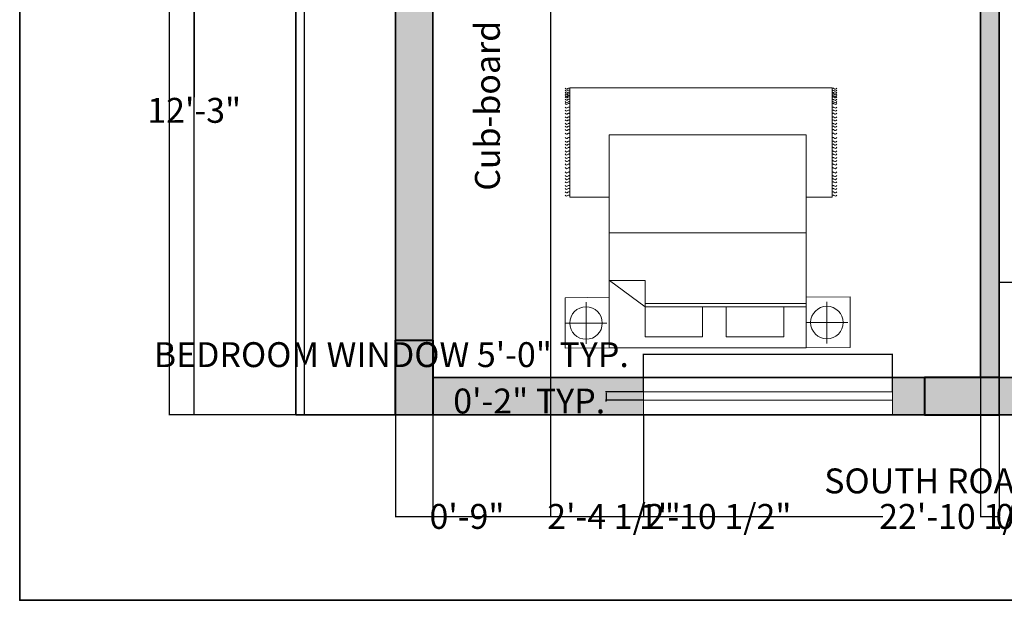
# Model space of a CAD drawing. Units: inches. Extents: x 56944 to 57417, y 173916 to 174454.
# Tile 1 of 8: x 56944 to 57181, y 173916 to 174056. Entities that reach past the tile are written whole.
import ezdxf

# ---------------------------------------------------------------- set-up
doc = ezdxf.new("R2010")
doc.units = ezdxf.units.IN
doc.header["$MEASUREMENT"] = 0
for name, color, linetype, lineweight in [('A-ANNO-DIMS', 2, 'Continuous', 18), ('A-ANNO-TEXT', 7, 'Continuous', 18), ('A-ANNO-TTLB', 7, 'Continuous', 35), ('A-COLS', 7, 'Continuous', 40), ('A-COLS-PATT', 250, 'Continuous', 9), ('A-FLOR-CASE', 8, 'Continuous', 25), ('A-FURN', 8, 'Continuous', 18), ('A-GLAZ', 4, 'Continuous', 18), ('A-SITE-PATT', 8, 'Continuous', 9), ('A-SITE-WALL', 7, 'Continuous', 25), ('A-WALL', 7, 'Continuous', 35), ('A-WALL-PATT', 241, 'Continuous', 9), ('C-PROP', 7, 'Continuous', 35)]:
    doc.layers.add(name, color=color, linetype=linetype, lineweight=lineweight)
doc.styles.get("Standard").update_dxf_attribs({"font": 'arial.ttf'})
doc.dimstyles.get("Standard").update_dxf_attribs({"dimtxt": 6, "dimasz": 0.18, "dimexe": 0.18, "dimexo": 0.0625, "dimgap": 0.09, "dimtad": 0, "dimtih": 1, "dimtoh": 1, "dimdec": 1, "dimzin": 0, "dimdsep": 46, "dimlunit": 3, "dimtxsty": 'Standard', "dimcen": 0.09, "dimadec": 0, "dimazin": 0, "dimtfac": 1, "dimtdec": 1, "dimtofl": 0, "dimtmove": 0, "dimatfit": 3, "dimfxl": 1, "dimtolj": 1, "dimtzin": 0, "dimarcsym": 0})

# ---------------------------------------------------------------- blocks, each defined once
blk = doc.blocks.new('*D4')
at = {"layer": 'A-ANNO-DIMS', "color": 0, "lineweight": -2, "transparency": 16777216}
for p, q in [((57010.07, 174399.82), (56979.48, 174399.82)), ((56979.66, 174399.64), (56979.66, 174183.23)), ((56979.66, 173960.5), (56979.66, 174176.92)), ((57010.07, 173960.32), (56979.48, 173960.32))]:
    blk.add_line(p, q, dxfattribs=at)
at = {"layer": 'A-ANNO-DIMS', "color": 0, "transparency": 16777216}
for points in [[(56979.63, 174399.64), (56979.69, 174399.64), (56979.66, 174399.82)], [(56979.63, 173960.5), (56979.69, 173960.5), (56979.66, 173960.32)]]:
    blk.add_solid(points, dxfattribs=at)
at = {"layer": 'Defpoints', "color": 0, "transparency": 16777216}
for p in [(57010.13, 174399.82), (56979.66, 173960.32), (57010.13, 173960.32)]:
    blk.add_point(p, dxfattribs=at)
at = {"layer": 'A-ANNO-DIMS', "color": 0, "transparency": 16777216, "insert": (56979.66, 174180.07), "char_height": 6, "width": 27.5975, "attachment_point": 5}
blk.add_mtext("\\A1;40'", dxfattribs=at)
blk = doc.blocks.new('BED-DOUBLE-WITH-NIGHTSTANDS')
for p, q in [((6.09, 68.68), (6.09, 58.62)), ((36.42, 67.59), (62.78, 67.59)), ((36.42, 58.05), (36.42, 67.59)), ((62.78, 67.59), (62.78, 4.35)), ((1.07, 63.65), (11.12, 63.65)), ((9.97, 49.39), (16.32, 58)), ((16.32, 49.44), (16.32, 58)), ((27.82, 58.05), (27.82, 10.63)), ((9.97, 49.44), (16.32, 49.44)), ((9.97, 49.39), (9.97, 10.63)), ((10.78, 49.44), (10.78, 10.63)), ((6.2, 10.63), (6.2, 0.57)), ((36.42, 4.35), (36.42, 10.65)), ((1.17, 5.6), (11.22, 5.6)), ((62.78, 4.35), (36.42, 4.35))]:
    blk.add_line(p, q)
for points in [[(12.29, 58.05), (12.19, 68.68), (0, 68.68), (0.1, 58.05)], [(0.1, 58.05), (51.42, 58.05), (51.42, 10.63), (0.1, 10.63)], [(2.8, 49.44), (9.97, 49.44), (9.97, 35.55), (2.8, 35.55)], [(2.8, 29.88), (9.97, 29.88), (9.97, 15.98), (2.8, 15.98)], [(12.39, 0), (12.29, 10.63), (0.1, 10.63), (0.21, 0)]]:
    blk.add_lwpolyline(points, close=True)
for centre in [(6.09, 63.65), (6.2, 5.6)]:
    blk.add_circle(centre, 3.92)
for points, knots in [([(36.95, 68.71), (36.83, 68.61), (36.59, 68.42), (36.83, 68.08), (37, 67.8), (36.89, 67.65), (36.85, 67.58)], [0, 0, 0, 0, 0.400747, 0.791423, 1.067667, 1.29709, 1.29709, 1.29709, 1.29709]), ([(37.73, 68.71), (37.61, 68.61), (37.37, 68.42), (37.61, 68.08), (37.78, 67.8), (37.67, 67.65), (37.62, 67.58)], [0, 0, 0, 0, 0.400747, 0.791423, 1.067667, 1.29709, 1.29709, 1.29709, 1.29709]), ([(38.54, 68.71), (38.42, 68.61), (38.18, 68.42), (38.42, 68.08), (38.59, 67.8), (38.49, 67.65), (38.44, 67.58)], [0, 0, 0, 0, 0.400747, 0.791423, 1.067667, 1.29709, 1.29709, 1.29709, 1.29709]), ([(39.27, 68.71), (39.15, 68.61), (38.91, 68.42), (39.15, 68.08), (39.32, 67.8), (39.22, 67.65), (39.17, 67.58)], [0, 0, 0, 0, 0.400747, 0.791423, 1.067667, 1.29709, 1.29709, 1.29709, 1.29709]), ([(40.15, 68.71), (40.03, 68.61), (39.79, 68.42), (40.03, 68.08), (40.2, 67.8), (40.1, 67.65), (40.05, 67.58)], [0, 0, 0, 0, 0.400747, 0.791423, 1.067667, 1.29709, 1.29709, 1.29709, 1.29709]), ([(40.91, 68.71), (40.78, 68.61), (40.54, 68.42), (40.78, 68.08), (40.96, 67.8), (40.85, 67.65), (40.8, 67.58)], [0, 0, 0, 0, 0.400747, 0.791423, 1.067667, 1.29709, 1.29709, 1.29709, 1.29709]), ([(41.63, 68.71), (41.51, 68.61), (41.27, 68.42), (41.51, 68.08), (41.68, 67.8), (41.58, 67.65), (41.53, 67.58)], [0, 0, 0, 0, 0.400747, 0.791423, 1.067667, 1.29709, 1.29709, 1.29709, 1.29709]), ([(42.52, 68.71), (42.39, 68.61), (42.15, 68.42), (42.39, 68.08), (42.57, 67.8), (42.46, 67.65), (42.41, 67.58)], [0, 0, 0, 0, 0.400747, 0.791423, 1.067667, 1.29709, 1.29709, 1.29709, 1.29709]), ([(43.55, 68.71), (43.43, 68.61), (43.19, 68.42), (43.43, 68.08), (43.6, 67.8), (43.5, 67.65), (43.45, 67.58)], [0, 0, 0, 0, 0.400747, 0.791423, 1.067667, 1.29709, 1.29709, 1.29709, 1.29709]), ([(44.43, 68.71), (44.31, 68.61), (44.07, 68.42), (44.31, 68.08), (44.49, 67.8), (44.38, 67.65), (44.33, 67.58)], [0, 0, 0, 0, 0.400747, 0.791423, 1.067667, 1.29709, 1.29709, 1.29709, 1.29709]), ([(45.25, 68.71), (45.13, 68.61), (44.89, 68.42), (45.13, 68.08), (45.3, 67.8), (45.2, 67.65), (45.15, 67.58)], [0, 0, 0, 0, 0.400747, 0.791423, 1.067667, 1.29709, 1.29709, 1.29709, 1.29709]), ([(46.03, 68.71), (45.91, 68.61), (45.67, 68.42), (45.91, 68.08), (46.08, 67.8), (45.97, 67.65), (45.92, 67.58)], [0, 0, 0, 0, 0.400747, 0.791423, 1.067667, 1.29709, 1.29709, 1.29709, 1.29709]), ([(46.84, 68.71), (46.72, 68.61), (46.48, 68.42), (46.72, 68.08), (46.9, 67.8), (46.79, 67.65), (46.74, 67.58)], [0, 0, 0, 0, 0.400747, 0.791423, 1.067667, 1.29709, 1.29709, 1.29709, 1.29709]), ([(47.57, 68.71), (47.45, 68.61), (47.21, 68.42), (47.45, 68.08), (47.62, 67.8), (47.52, 67.65), (47.47, 67.58)], [0, 0, 0, 0, 0.400747, 0.791423, 1.067667, 1.29709, 1.29709, 1.29709, 1.29709]), ([(48.45, 68.71), (48.33, 68.61), (48.09, 68.42), (48.33, 68.08), (48.51, 67.8), (48.4, 67.65), (48.35, 67.58)], [0, 0, 0, 0, 0.400747, 0.791423, 1.067667, 1.29709, 1.29709, 1.29709, 1.29709]), ([(49.21, 68.71), (49.08, 68.61), (48.85, 68.42), (49.08, 68.08), (49.26, 67.8), (49.15, 67.65), (49.1, 67.58)], [0, 0, 0, 0, 0.400747, 0.791423, 1.067667, 1.29709, 1.29709, 1.29709, 1.29709]), ([(49.93, 68.71), (49.81, 68.61), (49.57, 68.42), (49.81, 68.08), (49.99, 67.8), (49.88, 67.65), (49.83, 67.58)], [0, 0, 0, 0, 0.400747, 0.791423, 1.067667, 1.29709, 1.29709, 1.29709, 1.29709]), ([(50.82, 68.71), (50.69, 68.61), (50.46, 68.42), (50.69, 68.08), (50.87, 67.8), (50.76, 67.65), (50.71, 67.58)], [0, 0, 0, 0, 0.400747, 0.791423, 1.067667, 1.29709, 1.29709, 1.29709, 1.29709]), ([(51.85, 68.71), (51.73, 68.61), (51.49, 68.42), (51.73, 68.08), (51.9, 67.8), (51.8, 67.65), (51.75, 67.58)], [0, 0, 0, 0, 0.400747, 0.791423, 1.067667, 1.29709, 1.29709, 1.29709, 1.29709]), ([(52.73, 68.71), (52.61, 68.61), (52.37, 68.42), (52.61, 68.08), (52.79, 67.8), (52.68, 67.65), (52.63, 67.58)], [0, 0, 0, 0, 0.400747, 0.791423, 1.067667, 1.29709, 1.29709, 1.29709, 1.29709]), ([(53.55, 68.71), (53.43, 68.61), (53.19, 68.42), (53.43, 68.08), (53.6, 67.8), (53.5, 67.65), (53.45, 67.58)], [0, 0, 0, 0, 0.400747, 0.791423, 1.067667, 1.29709, 1.29709, 1.29709, 1.29709]), ([(54.24, 68.71), (54.12, 68.61), (53.88, 68.42), (54.12, 68.08), (54.29, 67.8), (54.19, 67.65), (54.14, 67.58)], [0, 0, 0, 0, 0.400747, 0.791423, 1.067667, 1.29709, 1.29709, 1.29709, 1.29709]), ([(55.06, 68.71), (54.94, 68.61), (54.7, 68.42), (54.94, 68.08), (55.11, 67.8), (55, 67.65), (54.95, 67.58)], [0, 0, 0, 0, 0.400747, 0.791423, 1.067667, 1.29709, 1.29709, 1.29709, 1.29709]), ([(55.78, 68.71), (55.66, 68.61), (55.42, 68.42), (55.66, 68.08), (55.84, 67.8), (55.73, 67.65), (55.68, 67.58)], [0, 0, 0, 0, 0.400747, 0.791423, 1.067667, 1.29709, 1.29709, 1.29709, 1.29709]), ([(56.67, 68.71), (56.55, 68.61), (56.31, 68.42), (56.55, 68.08), (56.72, 67.8), (56.61, 67.65), (56.56, 67.58)], [0, 0, 0, 0, 0.400747, 0.791423, 1.067667, 1.29709, 1.29709, 1.29709, 1.29709]), ([(57.42, 68.71), (57.3, 68.61), (57.06, 68.42), (57.3, 68.08), (57.47, 67.8), (57.36, 67.65), (57.32, 67.58)], [0, 0, 0, 0, 0.400747, 0.791423, 1.067667, 1.29709, 1.29709, 1.29709, 1.29709]), ([(58.15, 68.71), (58.03, 68.61), (57.79, 68.42), (58.03, 68.08), (58.2, 67.8), (58.1, 67.66), (58.05, 67.59)], [0, 0, 0, 0, 0.400747, 0.791423, 1.067667, 1.283686, 1.283686, 1.283686, 1.283686]), ([(59.03, 68.71), (58.91, 68.61), (58.67, 68.42), (58.91, 68.08), (59.08, 67.8), (58.98, 67.66), (58.93, 67.59)], [0, 0, 0, 0, 0.400747, 0.791423, 1.067667, 1.283686, 1.283686, 1.283686, 1.283686]), ([(59.46, 68.71), (59.34, 68.61), (59.09, 68.42), (59.34, 68.08), (59.51, 67.8), (59.41, 67.66), (59.36, 67.59)], [0, 0, 0, 0, 0.402903, 0.794912, 1.071156, 1.287177, 1.287177, 1.287177, 1.287177]), ([(60.05, 68.71), (59.93, 68.61), (59.69, 68.42), (59.93, 68.08), (60.1, 67.8), (60, 67.66), (59.96, 67.59)], [0, 0, 0, 0, 0.400747, 0.791423, 1.067667, 1.283686, 1.283686, 1.283686, 1.283686]), ([(60.63, 68.71), (60.51, 68.61), (60.27, 68.42), (60.51, 68.08), (60.68, 67.8), (60.58, 67.66), (60.53, 67.59)], [0, 0, 0, 0, 0.400747, 0.791423, 1.067667, 1.283686, 1.283686, 1.283686, 1.283686]), ([(60.94, 68.71), (60.82, 68.61), (60.58, 68.42), (60.81, 68.08), (60.99, 67.8), (60.89, 67.66), (60.84, 67.59)], [0, 0, 0, 0, 0.400747, 0.791423, 1.067667, 1.283686, 1.283686, 1.283686, 1.283686]), ([(61.35, 68.71), (61.23, 68.61), (60.99, 68.42), (61.23, 68.08), (61.41, 67.8), (61.3, 67.65), (61.25, 67.58)], [0, 0, 0, 0, 0.400747, 0.791423, 1.067667, 1.29709, 1.29709, 1.29709, 1.29709]), ([(61.75, 68.71), (61.63, 68.61), (61.39, 68.42), (61.63, 68.08), (61.8, 67.8), (61.7, 67.65), (61.65, 67.58)], [0, 0, 0, 0, 0.400747, 0.791423, 1.067667, 1.29709, 1.29709, 1.29709, 1.29709]), ([(62.24, 68.71), (62.12, 68.61), (61.88, 68.42), (62.12, 68.08), (62.29, 67.8), (62.18, 67.65), (62.13, 67.58)], [0, 0, 0, 0, 0.400747, 0.791423, 1.067667, 1.29709, 1.29709, 1.29709, 1.29709]), ([(62.71, 68.71), (62.59, 68.61), (62.35, 68.42), (62.59, 68.08), (62.76, 67.8), (62.66, 67.65), (62.61, 67.58)], [0, 0, 0, 0, 0.400747, 0.791423, 1.067667, 1.29709, 1.29709, 1.29709, 1.29709]), ([(36.95, 3.23), (36.83, 3.32), (36.59, 3.52), (36.83, 3.86), (37, 4.14), (36.89, 4.29), (36.85, 4.35)], [0, 0, 0, 0, 0.400747, 0.791423, 1.067667, 1.29709, 1.29709, 1.29709, 1.29709]), ([(37.73, 3.23), (37.61, 3.32), (37.37, 3.52), (37.61, 3.86), (37.78, 4.14), (37.67, 4.29), (37.62, 4.35)], [0, 0, 0, 0, 0.400747, 0.791423, 1.067667, 1.29709, 1.29709, 1.29709, 1.29709]), ([(38.54, 3.23), (38.42, 3.32), (38.18, 3.52), (38.42, 3.86), (38.59, 4.14), (38.49, 4.29), (38.44, 4.35)], [0, 0, 0, 0, 0.400747, 0.791423, 1.067667, 1.29709, 1.29709, 1.29709, 1.29709]), ([(39.27, 3.23), (39.15, 3.32), (38.91, 3.52), (39.15, 3.86), (39.32, 4.14), (39.22, 4.29), (39.17, 4.35)], [0, 0, 0, 0, 0.400747, 0.791423, 1.067667, 1.29709, 1.29709, 1.29709, 1.29709]), ([(40.15, 3.23), (40.03, 3.32), (39.79, 3.52), (40.03, 3.86), (40.2, 4.14), (40.1, 4.29), (40.05, 4.35)], [0, 0, 0, 0, 0.400747, 0.791423, 1.067667, 1.29709, 1.29709, 1.29709, 1.29709]), ([(40.91, 3.23), (40.78, 3.32), (40.54, 3.52), (40.78, 3.86), (40.96, 4.14), (40.85, 4.29), (40.8, 4.35)], [0, 0, 0, 0, 0.400747, 0.791423, 1.067667, 1.29709, 1.29709, 1.29709, 1.29709]), ([(41.63, 3.23), (41.51, 3.32), (41.27, 3.52), (41.51, 3.86), (41.68, 4.14), (41.58, 4.29), (41.53, 4.35)], [0, 0, 0, 0, 0.400747, 0.791423, 1.067667, 1.29709, 1.29709, 1.29709, 1.29709]), ([(42.52, 3.23), (42.39, 3.32), (42.15, 3.52), (42.39, 3.86), (42.57, 4.14), (42.46, 4.29), (42.41, 4.35)], [0, 0, 0, 0, 0.400747, 0.791423, 1.067667, 1.29709, 1.29709, 1.29709, 1.29709]), ([(43.55, 3.23), (43.43, 3.32), (43.19, 3.52), (43.43, 3.86), (43.6, 4.14), (43.5, 4.29), (43.45, 4.35)], [0, 0, 0, 0, 0.400747, 0.791423, 1.067667, 1.29709, 1.29709, 1.29709, 1.29709]), ([(44.43, 3.23), (44.31, 3.32), (44.07, 3.52), (44.31, 3.86), (44.49, 4.14), (44.38, 4.29), (44.33, 4.35)], [0, 0, 0, 0, 0.400747, 0.791423, 1.067667, 1.29709, 1.29709, 1.29709, 1.29709]), ([(45.25, 3.23), (45.13, 3.32), (44.89, 3.52), (45.13, 3.86), (45.3, 4.14), (45.2, 4.29), (45.15, 4.35)], [0, 0, 0, 0, 0.400747, 0.791423, 1.067667, 1.29709, 1.29709, 1.29709, 1.29709]), ([(46.03, 3.23), (45.91, 3.32), (45.67, 3.52), (45.91, 3.86), (46.08, 4.14), (45.97, 4.29), (45.92, 4.35)], [0, 0, 0, 0, 0.400747, 0.791423, 1.067667, 1.29709, 1.29709, 1.29709, 1.29709]), ([(46.84, 3.23), (46.72, 3.32), (46.48, 3.52), (46.72, 3.86), (46.9, 4.14), (46.79, 4.29), (46.74, 4.35)], [0, 0, 0, 0, 0.400747, 0.791423, 1.067667, 1.29709, 1.29709, 1.29709, 1.29709]), ([(47.57, 3.23), (47.45, 3.32), (47.21, 3.52), (47.45, 3.86), (47.62, 4.14), (47.52, 4.29), (47.47, 4.35)], [0, 0, 0, 0, 0.400747, 0.791423, 1.067667, 1.29709, 1.29709, 1.29709, 1.29709]), ([(48.45, 3.23), (48.33, 3.32), (48.09, 3.52), (48.33, 3.86), (48.51, 4.14), (48.4, 4.29), (48.35, 4.35)], [0, 0, 0, 0, 0.400747, 0.791423, 1.067667, 1.29709, 1.29709, 1.29709, 1.29709]), ([(49.21, 3.23), (49.08, 3.32), (48.85, 3.52), (49.08, 3.86), (49.26, 4.14), (49.15, 4.29), (49.1, 4.35)], [0, 0, 0, 0, 0.400747, 0.791423, 1.067667, 1.29709, 1.29709, 1.29709, 1.29709]), ([(49.93, 3.23), (49.81, 3.32), (49.57, 3.52), (49.81, 3.86), (49.99, 4.14), (49.88, 4.29), (49.83, 4.35)], [0, 0, 0, 0, 0.400747, 0.791423, 1.067667, 1.29709, 1.29709, 1.29709, 1.29709]), ([(50.82, 3.23), (50.69, 3.32), (50.46, 3.52), (50.69, 3.86), (50.87, 4.14), (50.76, 4.29), (50.71, 4.35)], [0, 0, 0, 0, 0.400747, 0.791423, 1.067667, 1.29709, 1.29709, 1.29709, 1.29709]), ([(51.85, 3.23), (51.73, 3.32), (51.49, 3.52), (51.73, 3.86), (51.9, 4.14), (51.8, 4.29), (51.75, 4.35)], [0, 0, 0, 0, 0.400747, 0.791423, 1.067667, 1.29709, 1.29709, 1.29709, 1.29709]), ([(52.73, 3.23), (52.61, 3.32), (52.37, 3.52), (52.61, 3.86), (52.79, 4.14), (52.68, 4.29), (52.63, 4.35)], [0, 0, 0, 0, 0.400747, 0.791423, 1.067667, 1.29709, 1.29709, 1.29709, 1.29709]), ([(53.55, 3.23), (53.43, 3.32), (53.19, 3.52), (53.43, 3.86), (53.6, 4.14), (53.5, 4.29), (53.45, 4.35)], [0, 0, 0, 0, 0.400747, 0.791423, 1.067667, 1.29709, 1.29709, 1.29709, 1.29709]), ([(54.24, 3.23), (54.12, 3.32), (53.88, 3.52), (54.12, 3.86), (54.29, 4.14), (54.19, 4.29), (54.14, 4.35)], [0, 0, 0, 0, 0.400747, 0.791423, 1.067667, 1.29709, 1.29709, 1.29709, 1.29709]), ([(55.06, 3.23), (54.94, 3.32), (54.7, 3.52), (54.94, 3.86), (55.11, 4.14), (55, 4.29), (54.95, 4.35)], [0, 0, 0, 0, 0.400747, 0.791423, 1.067667, 1.29709, 1.29709, 1.29709, 1.29709]), ([(55.78, 3.23), (55.66, 3.32), (55.42, 3.52), (55.66, 3.86), (55.84, 4.14), (55.73, 4.29), (55.68, 4.35)], [0, 0, 0, 0, 0.400747, 0.791423, 1.067667, 1.29709, 1.29709, 1.29709, 1.29709]), ([(56.67, 3.23), (56.55, 3.32), (56.31, 3.52), (56.55, 3.86), (56.72, 4.14), (56.61, 4.29), (56.56, 4.35)], [0, 0, 0, 0, 0.400747, 0.791423, 1.067667, 1.29709, 1.29709, 1.29709, 1.29709]), ([(57.42, 3.23), (57.3, 3.32), (57.06, 3.52), (57.3, 3.86), (57.47, 4.14), (57.36, 4.29), (57.32, 4.35)], [0, 0, 0, 0, 0.400747, 0.791423, 1.067667, 1.29709, 1.29709, 1.29709, 1.29709]), ([(58.15, 3.23), (58.03, 3.32), (57.79, 3.52), (58.03, 3.86), (58.2, 4.14), (58.09, 4.29), (58.04, 4.35)], [0, 0, 0, 0, 0.400747, 0.791423, 1.067667, 1.29709, 1.29709, 1.29709, 1.29709]), ([(59.03, 3.23), (58.91, 3.32), (58.67, 3.52), (58.91, 3.86), (59.08, 4.14), (58.97, 4.29), (58.93, 4.35)], [0, 0, 0, 0, 0.400747, 0.791423, 1.067667, 1.29709, 1.29709, 1.29709, 1.29709]), ([(59.46, 3.23), (59.33, 3.32), (59.08, 3.51), (59.34, 3.86), (59.51, 4.14), (59.4, 4.29), (59.36, 4.35)], [0, 0, 0, 0, 0.407265, 0.802015, 1.07826, 1.307683, 1.307683, 1.307683, 1.307683]), ([(60.03, 3.23), (59.9, 3.32), (59.67, 3.52), (59.9, 3.86), (60.08, 4.14), (59.97, 4.29), (59.92, 4.35)], [0, 0, 0, 0, 0.400747, 0.791423, 1.067667, 1.29709, 1.29709, 1.29709, 1.29709]), ([(60.6, 3.23), (60.48, 3.32), (60.24, 3.52), (60.48, 3.86), (60.65, 4.14), (60.54, 4.29), (60.5, 4.35)], [0, 0, 0, 0, 0.400747, 0.791423, 1.067667, 1.29709, 1.29709, 1.29709, 1.29709]), ([(60.91, 3.23), (60.79, 3.32), (60.55, 3.52), (60.79, 3.86), (60.96, 4.14), (60.85, 4.29), (60.81, 4.35)], [0, 0, 0, 0, 0.400747, 0.791423, 1.067667, 1.29709, 1.29709, 1.29709, 1.29709]), ([(61.33, 3.23), (61.21, 3.32), (60.97, 3.52), (61.21, 3.86), (61.38, 4.14), (61.27, 4.29), (61.22, 4.35)], [0, 0, 0, 0, 0.400747, 0.791423, 1.067667, 1.29709, 1.29709, 1.29709, 1.29709]), ([(61.72, 3.23), (61.6, 3.32), (61.36, 3.52), (61.6, 3.86), (61.78, 4.14), (61.67, 4.29), (61.62, 4.35)], [0, 0, 0, 0, 0.400747, 0.791423, 1.067667, 1.29709, 1.29709, 1.29709, 1.29709]), ([(62.21, 3.23), (62.09, 3.32), (61.85, 3.52), (62.09, 3.86), (62.26, 4.14), (62.15, 4.29), (62.11, 4.35)], [0, 0, 0, 0, 0.400747, 0.791423, 1.067667, 1.29709, 1.29709, 1.29709, 1.29709]), ([(62.71, 3.23), (62.59, 3.32), (62.35, 3.52), (62.59, 3.86), (62.76, 4.14), (62.66, 4.29), (62.61, 4.35)], [0, 0, 0, 0, 0.400747, 0.791423, 1.067667, 1.29709, 1.29709, 1.29709, 1.29709])]:
    blk.add_open_spline(points, degree=3, knots=knots)
blk = doc.blocks.new('GLAZ-LITE-60IN')
for p, q in [((0, 2), (60, 2)), ((60, 0), (0, 0))]:
    blk.add_line(p, q)
blk = doc.blocks.new('*D26')
at = {"layer": 'A-ANNO-DIMS', "color": 0, "lineweight": -2, "transparency": 16777216}
for p, q in [((57093.93, 173974.82), (57093.75, 173974.82)), ((57093.93, 173965.89), (57093.93, 173975)), ((57153.75, 173974.82), (57094.11, 173974.82)), ((57153.93, 173965.89), (57153.93, 173975))]:
    blk.add_line(p, q, dxfattribs=at)
at = {"layer": 'A-ANNO-DIMS', "color": 0, "transparency": 16777216}
for points in [[(57094.11, 173974.85), (57094.11, 173974.79), (57093.93, 173974.82)], [(57153.75, 173974.85), (57153.75, 173974.79), (57153.93, 173974.82)]]:
    blk.add_solid(points, dxfattribs=at)
at = {"layer": 'Defpoints', "color": 0, "transparency": 16777216}
for p in [(57093.93, 173974.82), (57093.93, 173965.82), (57153.93, 173965.82)]:
    blk.add_point(p, dxfattribs=at)
at = {"layer": 'A-ANNO-DIMS', "color": 0, "transparency": 16777216, "insert": (57033.14, 173974.82), "char_height": 6, "attachment_point": 5}
blk.add_mtext('\\A1;BEDROOM WINDOW 5\'-0" TYP.', dxfattribs=at)
blk = doc.blocks.new('*D27')
at = {"layer": 'A-ANNO-DIMS', "color": 0, "lineweight": -2, "transparency": 16777216}
for p, q in [((57093.87, 173965.82), (57084.75, 173965.82)), ((57084.93, 173965.64), (57084.93, 173964)), ((57093.87, 173963.82), (57084.75, 173963.82)), ((57084.93, 173963.64), (57084.75, 173963.64)), ((57084.93, 173963.82), (57084.93, 173963.64))]:
    blk.add_line(p, q, dxfattribs=at)
at = {"layer": 'A-ANNO-DIMS', "color": 0, "transparency": 16777216}
for points in [[(57084.9, 173965.64), (57084.96, 173965.64), (57084.93, 173965.82)], [(57084.9, 173964), (57084.96, 173964), (57084.93, 173963.82)]]:
    blk.add_solid(points, dxfattribs=at)
at = {"layer": 'Defpoints', "color": 0, "transparency": 16777216}
for p in [(57093.93, 173965.82), (57084.93, 173963.82), (57093.93, 173963.82)]:
    blk.add_point(p, dxfattribs=at)
at = {"layer": 'A-ANNO-DIMS', "color": 0, "transparency": 16777216, "insert": (57066.38, 173963.64), "char_height": 6, "attachment_point": 5}
blk.add_mtext('\\A1;0\'-2" TYP.', dxfattribs=at)
blk = doc.blocks.new('*D36')
at = {"layer": 'A-ANNO-DIMS', "color": 0, "lineweight": -2, "transparency": 16777216}
for p, q in [((57034.13, 173960.26), (57034.13, 173935.64)), ((57308.63, 173960.26), (57308.63, 173935.64)), ((57034.31, 173935.82), (57151.61, 173935.82)), ((57308.45, 173935.82), (57191.15, 173935.82))]:
    blk.add_line(p, q, dxfattribs=at)
at = {"layer": 'A-ANNO-DIMS', "color": 0, "transparency": 16777216}
for points in [[(57034.31, 173935.85), (57034.31, 173935.79), (57034.13, 173935.82)], [(57308.45, 173935.85), (57308.45, 173935.79), (57308.63, 173935.82)]]:
    blk.add_solid(points, dxfattribs=at)
at = {"layer": 'Defpoints', "color": 0, "transparency": 16777216}
for p in [(57034.13, 173960.32), (57308.63, 173960.32), (57308.63, 173935.82)]:
    blk.add_point(p, dxfattribs=at)
at = {"layer": 'A-ANNO-DIMS', "color": 0, "transparency": 16777216, "insert": (57171.38, 173935.82), "char_height": 6, "attachment_point": 5}
blk.add_mtext('\\A1;22\'-10 1/2"', dxfattribs=at)
blk = doc.blocks.new('*D37')
at = {"layer": 'A-ANNO-DIMS', "color": 0, "lineweight": -2, "transparency": 16777216}
for p, q in [((57034.07, 174321.82), (56985.45, 174321.82)), ((56985.63, 174321.64), (56985.63, 174144.27)), ((56985.63, 173960.5), (56985.63, 174137.88)), ((57034.07, 173960.32), (56985.45, 173960.32))]:
    blk.add_line(p, q, dxfattribs=at)
at = {"layer": 'A-ANNO-DIMS', "color": 0, "transparency": 16777216}
for points in [[(56985.6, 174321.64), (56985.66, 174321.64), (56985.63, 174321.82)], [(56985.6, 173960.5), (56985.66, 173960.5), (56985.63, 173960.32)]]:
    blk.add_solid(points, dxfattribs=at)
at = {"layer": 'Defpoints', "color": 0, "transparency": 16777216}
for p in [(56985.63, 174321.82), (57034.13, 174321.82), (57034.13, 173960.32)]:
    blk.add_point(p, dxfattribs=at)
at = {"layer": 'A-ANNO-DIMS', "color": 0, "transparency": 16777216, "insert": (56985.63, 174141.07), "char_height": 6, "attachment_point": 5}
blk.add_mtext('\\A1;30\'-1 1/2"', dxfattribs=at)
blk = doc.blocks.new('*D41')
at = {"layer": 'A-ANNO-DIMS', "color": 0, "lineweight": -2, "transparency": 16777216}
for p, q in [((57043.13, 173969.26), (57043.13, 173935.64)), ((57071.54, 173969.26), (57071.54, 173935.64)), ((57043.31, 173935.82), (57071.36, 173935.82)), ((57071.54, 173935.82), (57071.72, 173935.82))]:
    blk.add_line(p, q, dxfattribs=at)
at = {"layer": 'A-ANNO-DIMS', "color": 0, "transparency": 16777216}
for points in [[(57043.31, 173935.85), (57043.31, 173935.79), (57043.13, 173935.82)], [(57071.36, 173935.85), (57071.36, 173935.79), (57071.54, 173935.82)]]:
    blk.add_solid(points, dxfattribs=at)
at = {"layer": 'Defpoints', "color": 0, "transparency": 16777216}
for p in [(57043.13, 173969.32), (57071.54, 173969.32), (57071.54, 173935.82)]:
    blk.add_point(p, dxfattribs=at)
at = {"layer": 'A-ANNO-DIMS', "color": 0, "transparency": 16777216, "insert": (57086.83, 173935.82), "char_height": 6, "attachment_point": 5}
blk.add_mtext('\\A1;2\'-4 1/2"', dxfattribs=at)
blk = doc.blocks.new('*D47')
at = {"layer": 'A-ANNO-DIMS', "color": 0, "lineweight": -2, "transparency": 16777216}
for p, q in [((57034.13, 173960.26), (57034.13, 173935.64)), ((57043.13, 173960.26), (57043.13, 173935.64)), ((57034.31, 173935.82), (57042.95, 173935.82)), ((57043.13, 173935.82), (57043.31, 173935.82))]:
    blk.add_line(p, q, dxfattribs=at)
at = {"layer": 'A-ANNO-DIMS', "color": 0, "transparency": 16777216}
for points in [[(57034.31, 173935.85), (57034.31, 173935.79), (57034.13, 173935.82)], [(57042.95, 173935.85), (57042.95, 173935.79), (57043.13, 173935.82)]]:
    blk.add_solid(points, dxfattribs=at)
at = {"layer": 'Defpoints', "color": 0, "transparency": 16777216}
for p in [(57034.13, 173960.32), (57043.13, 173960.32), (57043.13, 173935.82)]:
    blk.add_point(p, dxfattribs=at)
at = {"layer": 'A-ANNO-DIMS', "color": 0, "transparency": 16777216, "insert": (57051.38, 173935.82), "char_height": 6, "attachment_point": 5}
blk.add_mtext('\\A1;0\'-9"', dxfattribs=at)
blk = doc.blocks.new('*D48')
at = {"layer": 'A-ANNO-DIMS', "color": 0, "lineweight": -2, "transparency": 16777216}
for p, q in [((57175.13, 173969.26), (57175.13, 173935.64)), ((57179.63, 173969.26), (57179.63, 173935.64)), ((57175.31, 173935.82), (57179.45, 173935.82)), ((57179.63, 173935.82), (57179.81, 173935.82))]:
    blk.add_line(p, q, dxfattribs=at)
at = {"layer": 'A-ANNO-DIMS', "color": 0, "transparency": 16777216}
for points in [[(57175.31, 173935.85), (57175.31, 173935.79), (57175.13, 173935.82)], [(57179.45, 173935.85), (57179.45, 173935.79), (57179.63, 173935.82)]]:
    blk.add_solid(points, dxfattribs=at)
at = {"layer": 'Defpoints', "color": 0, "transparency": 16777216}
for p in [(57175.13, 173969.32), (57179.63, 173969.32), (57179.63, 173935.82)]:
    blk.add_point(p, dxfattribs=at)
at = {"layer": 'A-ANNO-DIMS', "color": 0, "transparency": 16777216, "insert": (57194.87, 173935.82), "char_height": 6, "attachment_point": 5}
blk.add_mtext('\\A1;0\'-4 1/2"', dxfattribs=at)
blk = doc.blocks.new('*D58')
at = {"layer": 'A-ANNO-DIMS', "color": 0, "lineweight": -2, "transparency": 16777216}
for p, q in [((57071.54, 173969.26), (57071.54, 173935.64)), ((57093.93, 173960.26), (57093.93, 173935.64)), ((57071.72, 173935.82), (57093.75, 173935.82)), ((57093.93, 173935.82), (57094.11, 173935.82))]:
    blk.add_line(p, q, dxfattribs=at)
at = {"layer": 'A-ANNO-DIMS', "color": 0, "transparency": 16777216}
for points in [[(57071.72, 173935.85), (57071.72, 173935.79), (57071.54, 173935.82)], [(57093.75, 173935.85), (57093.75, 173935.79), (57093.93, 173935.82)]]:
    blk.add_solid(points, dxfattribs=at)
at = {"layer": 'Defpoints', "color": 0, "transparency": 16777216}
for p in [(57071.54, 173969.32), (57093.93, 173960.32), (57093.93, 173935.82)]:
    blk.add_point(p, dxfattribs=at)
at = {"layer": 'A-ANNO-DIMS', "color": 0, "transparency": 16777216, "insert": (57111.22, 173935.82), "char_height": 6, "attachment_point": 5}
blk.add_mtext('\\A1;1\'-10 1/2"', dxfattribs=at)
blk = doc.blocks.new('*D62')
at = {"layer": 'A-ANNO-DIMS', "color": 0, "lineweight": -2, "transparency": 16777216}
for p, q in [((57034.07, 174107.11), (56985.45, 174107.11)), ((56985.63, 174106.93), (56985.63, 174036.87)), ((56985.63, 173960.5), (56985.63, 174030.56)), ((57034.07, 173960.32), (56985.45, 173960.32))]:
    blk.add_line(p, q, dxfattribs=at)
at = {"layer": 'A-ANNO-DIMS', "color": 0, "transparency": 16777216}
for points in [[(56985.6, 174106.93), (56985.66, 174106.93), (56985.63, 174107.11)], [(56985.6, 173960.5), (56985.66, 173960.5), (56985.63, 173960.32)]]:
    blk.add_solid(points, dxfattribs=at)
at = {"layer": 'Defpoints', "color": 0, "transparency": 16777216}
for p in [(57034.13, 174107.11), (56985.63, 173960.32), (57034.13, 173960.32)]:
    blk.add_point(p, dxfattribs=at)
at = {"layer": 'A-ANNO-DIMS', "color": 0, "transparency": 16777216, "insert": (56985.63, 174033.71), "char_height": 6, "attachment_point": 5}
blk.add_mtext('\\A1;12\'-3"', dxfattribs=at)

msp = doc.modelspace()

# ---------------------------------------------------------------- hatches: boundary and pattern name
at = {"layer": 'A-COLS-PATT'}
h = msp.add_hatch(color=256, dxfattribs=at)
h.dxf.hatch_style = 1
h.paths.add_polyline_path([(57052.13, 174321.82), (57034.13, 174321.82), (57034.13, 174312.82), (57052.13, 174312.82)])
h.paths.add_polyline_path([(57186.38, 174321.82), (57168.38, 174321.82), (57168.38, 174312.82), (57175.13, 174312.82), (57186.38, 174312.82)])
h.paths.add_polyline_path([(57308.63, 174321.82), (57290.63, 174321.82), (57290.63, 174312.82), (57308.63, 174312.82)])
h.paths.add_polyline_path([(57179.63, 174204.82), (57170.63, 174204.82), (57170.63, 174186.82), (57179.63, 174186.82)])
h.paths.add_polyline_path([(57043.13, 174204.82), (57034.13, 174204.82), (57034.13, 174186.82), (57043.13, 174186.82)])
h.paths.add_polyline_path([(57308.63, 174206.32), (57299.63, 174206.32), (57299.63, 174188.32), (57308.63, 174188.32)])
h.paths.add_polyline_path([(57308.63, 174107.87), (57299.63, 174107.87), (57299.63, 174093.93), (57308.63, 174093.93)])
h.paths.add_polyline_path([(57308.63, 173978.32), (57299.63, 173978.32), (57299.63, 173960.32), (57308.63, 173960.32)])
h.paths.add_polyline_path([(57179.63, 173969.32), (57161.63, 173969.32), (57161.63, 173960.32), (57179.63, 173960.32)])
h.paths.add_polyline_path([(57043.13, 173978.32), (57034.13, 173978.32), (57034.13, 173960.32), (57043.13, 173960.32)])
h.paths.add_polyline_path([(57043.13, 174099.82), (57034.13, 174099.82), (57034.13, 174081.82), (57043.13, 174081.82)])
h.paths.add_polyline_path([(57179.63, 174099.82), (57170.63, 174099.82), (57170.63, 174081.82), (57179.63, 174081.82)])
at = {"layer": 'A-SITE-PATT'}
h = msp.add_hatch(dxfattribs=at)
h.set_pattern_fill('ANGLE', color=256, scale=50)
h.set_pattern_definition([(0, (0, 0), (0, 13.75), [10, -3.75]), (90, (0, 0), (-13.75, 8e-16), [10, -3.75])])
h.paths.add_polyline_path([(57365.63, 174396.82), (57200.13, 174396.82), (57200.13, 174379.18), (57215.46, 174379.18, -1.049383), (57218.84, 174379.34, -0.952941), (57215.46, 174379.18), (57200.13, 174379.18), (57200.13, 174360.82), (57140.13, 174360.82), (57140.13, 174321.82), (57149.42, 174321.82), (57243.2, 174321.82), (57282.32, 174321.82), (57283.32, 174321.82), (57308.63, 174321.82), (57308.63, 174305.82), (57308.63, 174259.72), (57308.63, 174258.72), (57308.63, 174252.72), (57308.63, 174216.72), (57308.63, 174099.82), (57308.63, 174093.93), (57308.63, 174081.93), (57308.63, 173969.32), (57365.63, 173969.32)])
h.paths.add_polyline_path([(57341.88, 174114.38), (57341.88, 174209.81), (57329.51, 174209.81), (57329.51, 174114.38)], flags=24)
h.paths.add_polyline_path([(57215.63, 174350.61), (57326.6, 174350.61), (57326.6, 174362.97), (57215.63, 174362.97)], flags=24)
at = {"layer": 'A-WALL-PATT'}
h = msp.add_hatch(color=256, dxfattribs=at)
h.dxf.hatch_style = 1
h.paths.add_polyline_path([(57089.42, 174321.82), (57052.13, 174321.82), (57052.13, 174312.82), (57089.42, 174312.82)])
h.paths.add_polyline_path([(57168.38, 174321.82), (57149.42, 174321.82), (57149.42, 174312.82), (57168.38, 174312.82)])
h.paths.add_polyline_path([(57199.66, 174321.82), (57186.38, 174321.82), (57186.38, 174312.82), (57199.66, 174312.82)])
h.paths.add_polyline_path([(57179.63, 174312.82), (57177.38, 174312.82), (57175.13, 174312.82), (57175.13, 174204.82), (57179.63, 174204.82)])
h.paths.add_polyline_path([(57043.13, 174312.82), (57034.13, 174312.82), (57034.13, 174204.82), (57043.13, 174204.82)])
h.paths.add_polyline_path([(57043.13, 174147.82), (57121.13, 174147.82), (57121.13, 174099.82), (57115.13, 174099.82), (57115.13, 174095.32), (57121.13, 174095.32), (57133.63, 174095.32), (57133.63, 174099.82), (57125.63, 174099.82), (57125.63, 174200.32), (57133.63, 174200.32), (57133.63, 174204.82), (57115.13, 174204.82), (57115.13, 174200.32), (57121.13, 174200.32), (57121.13, 174152.32), (57043.13, 174152.32), (57043.13, 174162.82), (57034.13, 174162.82), (57034.13, 174131.11), (57043.13, 174131.11)])
h.paths.add_polyline_path([(57043.13, 174081.82), (57034.13, 174081.82), (57034.13, 173978.32), (57043.13, 173978.32)])
h.paths.add_polyline_path([(57093.93, 173969.32), (57043.13, 173969.32), (57043.13, 173960.32), (57093.93, 173960.32)])
h.paths.add_polyline_path([(57161.63, 173969.32), (57153.93, 173969.32), (57153.93, 173960.32), (57161.63, 173960.32)])
h.paths.add_polyline_path([(57179.63, 174081.82), (57175.13, 174081.82), (57175.13, 173969.32), (57179.63, 173969.32)])
h.paths.add_polyline_path([(57299.63, 173969.32), (57179.63, 173969.32), (57179.63, 173960.32), (57299.63, 173960.32)])
h.paths.add_polyline_path([(57308.63, 174025.05), (57299.63, 174025.05), (57299.63, 173978.32), (57308.63, 173978.32)])
h.paths.add_polyline_path([(57308.63, 174081.93), (57299.63, 174081.93), (57299.63, 174075.82), (57227.63, 174075.82), (57227.63, 174081.82), (57223.13, 174081.82), (57223.13, 174075.82), (57223.13, 174071.32), (57299.63, 174071.32), (57299.63, 174061.05), (57308.63, 174061.05)])
h.paths.add_polyline_path([(57308.63, 174140.51), (57299.63, 174140.51), (57299.63, 174128.32), (57223.13, 174128.32), (57223.13, 174117.82), (57227.63, 174117.82), (57227.63, 174123.82), (57299.63, 174123.82), (57299.63, 174119.87), (57308.63, 174119.87)])
h.paths.add_polyline_path([(57308.63, 174216.72), (57299.63, 174216.72), (57299.63, 174206.32), (57308.63, 174206.32)])
h.paths.add_polyline_path([(57308.63, 174188.32), (57299.63, 174188.32), (57299.63, 174176.51), (57308.63, 174176.51)])
h.paths.add_polyline_path([(57308.63, 174258.72), (57299.63, 174258.72), (57299.63, 174252.72), (57308.63, 174252.72)])
h.paths.add_polyline_path([(57308.63, 174312.82), (57299.63, 174312.82), (57299.63, 174306.82), (57308.63, 174306.82)])
h.paths.add_polyline_path([(57290.63, 174321.82), (57283.32, 174321.82), (57283.32, 174312.82), (57290.63, 174312.82)])
h.paths.add_polyline_path([(57242.2, 174321.82), (57235.66, 174321.82), (57235.66, 174312.82), (57242.2, 174312.82)])
h.paths.add_polyline_path([(57083.13, 174204.82), (57043.13, 174204.82), (57043.13, 174200.32), (57083.13, 174200.32)], flags=17)
h.paths.add_polyline_path([(57083.13, 174099.82), (57043.13, 174099.82), (57043.13, 174095.32), (57083.13, 174095.32)], flags=0)

# ---------------------------------------------------------------- linework, layer by layer
at = {"layer": 'A-ANNO-TTLB'}
msp.add_lwpolyline([(56943.57, 174453.61), (57416.55, 174453.61), (57416.55, 173915.6), (56943.57, 173915.6)], close=True, dxfattribs=at)
at = {"layer": 'A-COLS'}
for p, q in [((57034.13, 173960.32), (57034.13, 173978.32)), ((57034.13, 173978.32), (57043.13, 173978.32)), ((57043.13, 173978.32), (57043.13, 173960.32)), ((57179.63, 173969.32), (57161.63, 173969.32)), ((57161.63, 173969.32), (57161.63, 173960.32)), ((57161.63, 173960.32), (57179.63, 173960.32))]:
    msp.add_line(p, q, dxfattribs=at)
at = {"layer": 'A-FLOR-CASE'}
for p, q in [((57071.54, 174095.32), (57071.54, 173969.32)), ((57273.2, 173992.24), (57179.63, 173992.24))]:
    msp.add_line(p, q, dxfattribs=at)
at = {"layer": 'A-GLAZ'}
for p, q in [((57093.93, 173960.32), (57093.93, 173969.32)), ((57093.93, 173969.32), (57153.93, 173969.32)), ((57153.93, 173969.32), (57153.93, 173960.32)), ((57153.93, 173960.32), (57093.93, 173960.32))]:
    msp.add_line(p, q, dxfattribs=at)
at = {"layer": 'A-SITE-WALL'}
msp.add_line((57012.13, 174397.82), (57012.13, 173960.32), dxfattribs=at)
at = {"layer": 'A-WALL'}
for p, q in [((57034.13, 174321.82), (57034.13, 173960.32)), ((57043.13, 174147.82), (57043.13, 173960.32)), ((57179.63, 174099.82), (57179.63, 173960.32)), ((57175.13, 174081.82), (57175.13, 173969.32)), ((57043.13, 173969.32), (57299.63, 173969.32)), ((57034.13, 173960.32), (57308.63, 173960.32))]:
    msp.add_line(p, q, dxfattribs=at)
at = {"layer": 'C-PROP'}
for p, q in [((57010.13, 174399.82), (57010.13, 173960.32)), ((57010.13, 173960.32), (57034.13, 173960.32))]:
    msp.add_line(p, q, dxfattribs=at)

# ---------------------------------------------------------------- block references
at = {"layer": 'A-FURN', "rotation": 90.00000000047704}
msp.add_blockref('BED-DOUBLE-WITH-NIGHTSTANDS', (57143.73, 173976.35), dxfattribs=at)
at = {"layer": 'A-GLAZ', "rotation": 180}
msp.add_blockref('GLAZ-LITE-60IN', (57153.93, 173965.82), dxfattribs=at)

# ---------------------------------------------------------------- texts
at = {"layer": 'A-ANNO-TEXT', "insert": (57053.3, 174014.34), "char_height": 6, "attachment_point": 1, "rotation": 90}
msp.add_mtext_dynamic_manual_height_columns('Cub-board ', width=64.2447, gutter_width=1, heights=[0], dxfattribs=at)
at = {"layer": 'A-ANNO-TEXT', "insert": (57137.49, 173947.38), "char_height": 6, "attachment_point": 1}
msp.add_mtext_dynamic_manual_height_columns('SOUTH ROAD ', width=99.0153, gutter_width=1, heights=[0], dxfattribs=at)

# ---------------------------------------------------------------- dimensions: what is measured, and where the dimension line sits
at = {"layer": 'A-ANNO-DIMS'}
for base, p1, p2, angle, text, override, picture, middle in [((56979.66, 173960.32), (57010.13, 174399.82), (57010.13, 173960.32), 90, "40'", {"dimclrd": 0, "dimclre": 0, "dimclrt": 0}, '*D4', (56979.66, 174180.07)), ((57093.93, 173974.82), (57153.93, 173965.82), (57093.93, 173965.82), 180, 'BEDROOM WINDOW <> TYP.', {"dimdec": 1, "dimlfac": 1, "dimrnd": 0, "dimzin": 1, "dimdsep": 46, "dimlunit": 4, "dimfrac": 2}, '*D26', (57033.14, 173974.82)), ((57084.93, 173963.82), (57093.93, 173965.82), (57093.93, 173963.82), 270, '<> TYP.', {"dimdec": 1, "dimlfac": 1, "dimrnd": 0, "dimzin": 1, "dimdsep": 46, "dimlunit": 4, "dimfrac": 2}, '*D27', (57066.38, 173963.64))]:
    dim = msp.add_linear_dim(base=base, p1=p1, p2=p2, angle=angle, text=text, dimstyle='Standard', override=override, dxfattribs=at)
    dim.commit()
    dim.dimension.update_dxf_attribs({"geometry": picture, "text_midpoint": middle})
for base, p1, p2, picture, middle in [((56985.63, 174321.82), (57034.13, 173960.32), (57034.13, 174321.82), '*D37', (56985.63, 174141.07)), ((56985.63, 173960.32), (57034.13, 174107.11), (57034.13, 173960.32), '*D62', (56985.63, 174033.71))]:
    dim = msp.add_linear_dim(base=base, p1=p1, p2=p2, angle=90, dimstyle='Standard', override={"dimdec": 1, "dimlfac": 1, "dimrnd": 0, "dimzin": 1, "dimdsep": 46, "dimlunit": 4, "dimfrac": 2}, dxfattribs=at)
    dim.commit()
    dim.dimension.update_dxf_attribs({"geometry": picture, "text_midpoint": middle})
for base, p1, p2, picture, middle in [((57071.54, 173935.82), (57043.13, 173969.32), (57071.54, 173969.32), '*D41', (57086.83, 173935.82)), ((57093.93, 173935.82), (57071.54, 173969.32), (57093.93, 173960.32), '*D58', (57111.22, 173935.82)), ((57179.63, 173935.82), (57175.13, 173969.32), (57179.63, 173969.32), '*D48', (57194.87, 173935.82)), ((57308.63, 173935.82), (57034.13, 173960.32), (57308.63, 173960.32), '*D36', (57171.38, 173935.82)), ((57043.13, 173935.82), (57034.13, 173960.32), (57043.13, 173960.32), '*D47', (57051.38, 173935.82))]:
    dim = msp.add_linear_dim(base=base, p1=p1, p2=p2, dimstyle='Standard', override={"dimdec": 1, "dimlfac": 1, "dimrnd": 0, "dimzin": 1, "dimdsep": 46, "dimlunit": 4, "dimfrac": 2}, dxfattribs=at)
    dim.commit()
    dim.dimension.update_dxf_attribs({"geometry": picture, "text_midpoint": middle})

doc.saveas('drawing.dxf')
